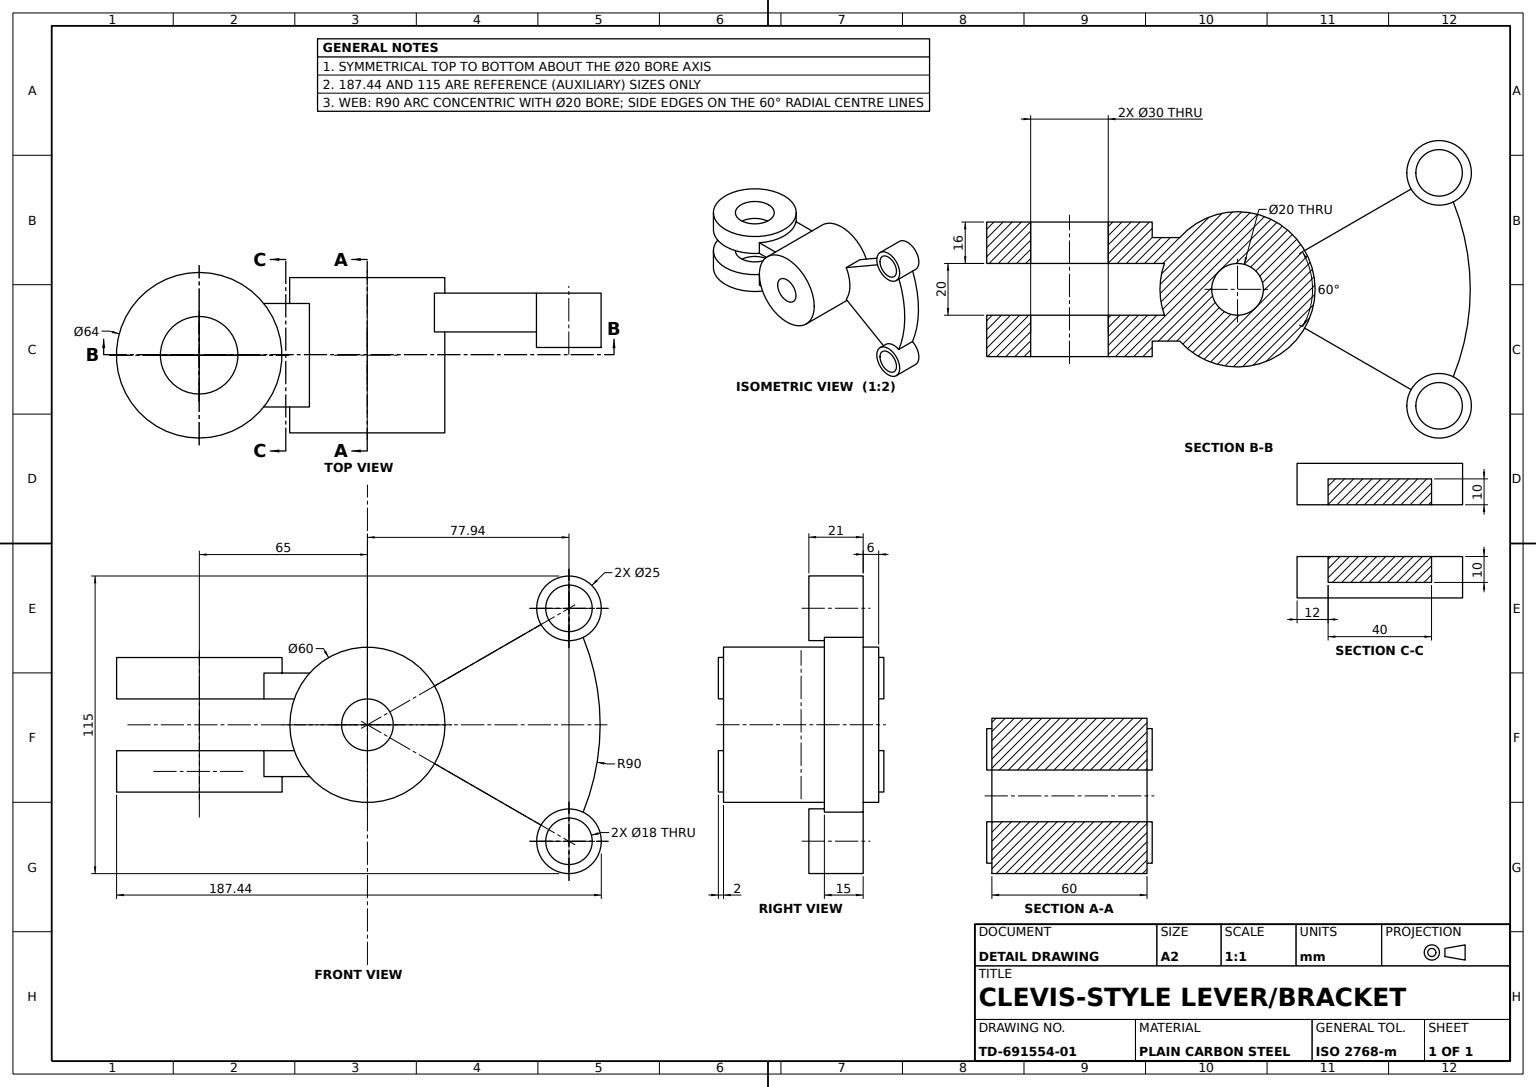
from build123d import *
from build123d.topology import SkipClean

# Parameters (mm, degrees)
HUB_SKETCH_R               = 30
HUB_60_DEPTH               = 60
MOUNTING_ARM_DEPTH         = 15
UPPER_LUG_BOSS_SKETCH_R    = 12.5
UPPER_LUG_BOSS_SKETCH_R_2  = 9
UPPER_LUG_BOSS_25_DEPTH    = 21
UPPER_LUG_HOLE_DEPTH       = 113.138562317
CLEVIS_ARM_DEPTH           = 10
CLEVIS_EYE_BOSS_SKETCH_R   = 32
CLEVIS_EYE_BOSS_SKETCH_R_2 = 15
CLEVIS_EYE_BOSS_DEPTH      = 16
CLEVIS_EYE_HOLE_SKETCH_R   = 15
CLEVIS_EYE_HOLE_DEPTH      = 136.255314129
HUB_BORE_SKETCH_R          = 10
HUB_BORE_20_DEPTH          = 129.682749427
LOWER_LUG_BOSS_SKETCH_R    = 12.5
LOWER_LUG_BOSS_SKETCH_R_2  = 9
LOWER_LUG_BOSS_DEPTH       = 21
LOWER_LUG_HOLE_DEPTH       = 120.984373983


with BuildPart() as part:
    # Hub Sketch → Hub Ø60 (new body)
    with BuildSketch(Plane.XY):
        Circle(HUB_SKETCH_R)
    extrude(amount=HUB_60_DEPTH)

    # Mounting Arm Sketch → Mounting Arm (add)
    with BuildSketch(Plane.XY.offset(6)):
        with BuildLine():
            Line((0, 0), (77.942286341, 45))
            ThreePointArc((77.942286341, 45), (90, 0), (77.942286341, -45))
            Line((77.942286341, -45), (0, 0))
        make_face()
    extrude(amount=MOUNTING_ARM_DEPTH)

    # Upper Lug Boss Sketch → Upper Lug Boss Ø25 (add)
    with BuildSketch(Plane.XY.offset(6)):
        with Locations(Location((77.942286341, 45, 0), (0, 0, 210))):
            Circle(UPPER_LUG_BOSS_SKETCH_R)
        with Locations(Location((77.942286341, 45, 0), (0, 0, 210))):
            Circle(UPPER_LUG_BOSS_SKETCH_R_2, mode=Mode.SUBTRACT)
    extrude(amount=UPPER_LUG_BOSS_25_DEPTH)

    # Upper Lug Hole Sketch → Upper Lug Hole (cut, through all)
    with BuildSketch(Plane.XY.offset(27)):
        with BuildLine():
            Line((70.148057707, 40.5), (80.210020809, 46.309277106))
            Line((80.210020809, 46.309277106), (84.515342337, 38.852241476))
            ThreePointArc((84.515342337, 38.852241476), (76.916814405, 36.058612674), (70.148057707, 40.5))
        make_face()
    extrude(amount=-UPPER_LUG_HOLE_DEPTH, mode=Mode.SUBTRACT)

    # Clevis Arm Sketch → Clevis Arm (add)
    with BuildSketch(Plane(origin=(0, 10, 0), x_dir=(1, 0, 0), z_dir=(0, 1, 0))):
        Polygon((-29.743772899, -10), (-22.043534858, -10), (-22.043534858, -50), (-30, -50), (-80, -50), (-80, -40), (-65, -40), (-65, -20), (-80, -20), (-80, -10), align=None)
    clevis_arm = extrude(amount=CLEVIS_ARM_DEPTH)

    # Clevis Arm Mirror: Clevis Arm across plane
    add(clevis_arm.mirror(Plane.ZX))

    # Clevis Eye Boss Sketch → Clevis Eye Boss (add)
    with BuildSketch(Plane(origin=(0, 10, 0), x_dir=(1, 0, 0), z_dir=(0, 1, 0))):
        with Locations(Location((-65, -30, 0), (0, 0, 38.682187453))):
            Circle(CLEVIS_EYE_BOSS_SKETCH_R)
        with Locations(Location((-65, -30, 0), (0, 0, 138.189685104))):
            Circle(CLEVIS_EYE_BOSS_SKETCH_R_2, mode=Mode.SUBTRACT)
    clevis_eye_boss = extrude(amount=CLEVIS_EYE_BOSS_DEPTH)

    # Clevis Eye Boss Mirror: Clevis Eye Boss across plane
    add(clevis_eye_boss.mirror(Plane.ZX))

    # Clevis Eye Hole Sketch → Clevis Eye Hole (cut, through all)
    with SkipClean():  # the faces are left unmerged after this step: merging them gives an invalid solid
        with BuildSketch(Plane(origin=(0, 26, 0), x_dir=(1, 0, 0), z_dir=(0, 1, 0))):
            with Locations(Location((-65, -30, 0), (0, 0, 270))):
                Circle(CLEVIS_EYE_HOLE_SKETCH_R)
        extrude(amount=-CLEVIS_EYE_HOLE_DEPTH, mode=Mode.SUBTRACT)

    # Hub Bore Sketch → Hub Bore Ø20 (cut, through all)
    with SkipClean():  # the faces are left unmerged after this step: merging them gives an invalid solid
        with BuildSketch(Plane.XY.offset(60)):
            Circle(HUB_BORE_SKETCH_R)
        extrude(amount=-HUB_BORE_20_DEPTH, mode=Mode.SUBTRACT)

    # Lower Lug Boss Sketch → Lower Lug Boss (add)
    with SkipClean():  # the faces are left unmerged after this step: merging them gives an invalid solid
        with BuildSketch(Plane.XY.offset(6)):
            with Locations(Location((77.942286341, -45, 0), (0, 0, 150))):
                Circle(LOWER_LUG_BOSS_SKETCH_R)
            with Locations(Location((77.942286341, -45, 0), (0, 0, 150))):
                Circle(LOWER_LUG_BOSS_SKETCH_R_2, mode=Mode.SUBTRACT)
        extrude(amount=LOWER_LUG_BOSS_DEPTH)

    # Lower Lug Hole Sketch → Lower Lug Hole (cut, through all)
    with SkipClean():  # the faces are left unmerged after this step: merging them gives an invalid solid
        with BuildSketch(Plane.XY.offset(21)):
            with BuildLine():
                Line((77.942286341, -45), (70.148057707, -40.5))
                ThreePointArc((70.148057707, -40.5), (75.396242131, -36.367638858), (82.046946389, -36.990520249))
                ThreePointArc((82.046946389, -36.990520249), (80.094797514, -41.046600483), (77.942286341, -45))
            make_face()
        extrude(amount=-LOWER_LUG_HOLE_DEPTH, mode=Mode.SUBTRACT)


solid = part.part
